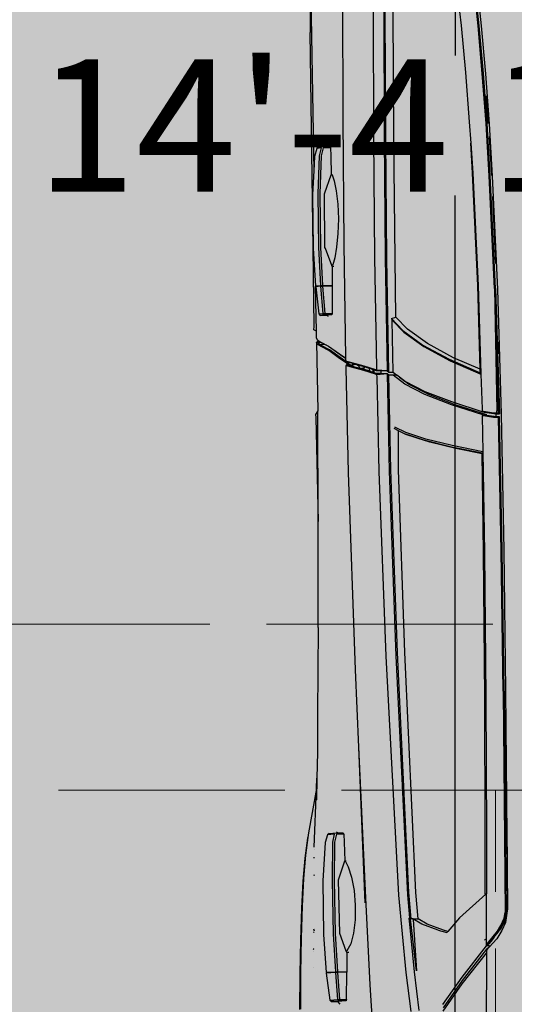
# Model space of a CAD drawing. Units: inches. Extents: x 1884 to 2398, y 474 to 1488.
# Tile 23 of 39: x 2275 to 2301, y 620 to 672. Entities that reach past the tile are written whole.
import ezdxf

# ---------------------------------------------------------------- set-up
doc = ezdxf.new("R2010")
doc.units = ezdxf.units.IN
doc.header["$MEASUREMENT"] = 0
doc.linetypes.add('ACAD_ISO02W100', pattern=[15, 12, -3])
doc.layers.get('0').update_dxf_attribs({"color": 250})
for name, color, linetype, lineweight in [('A-ANNO-DIMS', 2, 'Continuous', 18), ('A-FLOR-OVHD', 8, 'ACAD_ISO02W100', 18), ('C-VEHI', 8, 'Continuous', 18)]:
    doc.layers.add(name, color=color, linetype=linetype, lineweight=lineweight)
doc.layers.add('Edges', color=250, linetype='Continuous')
doc.layers.add('L-PVMT-PATT', color=9, linetype='Continuous', lineweight=13, true_color=0xc7c8ca)
doc.styles.get("Standard").update_dxf_attribs({"font": 'arial.ttf'})
doc.dimstyles.get("Standard").update_dxf_attribs({"dimtxt": 7, "dimasz": 0.18, "dimexe": 0.18, "dimexo": 0.0625, "dimgap": 0.09, "dimtad": 0, "dimtih": 1, "dimtoh": 1, "dimzin": 0, "dimdsep": 46, "dimlunit": 3, "dimtxsty": 'Standard', "dimcen": 0.09, "dimadec": 0, "dimazin": 0, "dimtfac": 1, "dimtofl": 0, "dimtmove": 0, "dimatfit": 3, "dimfxl": 1, "dimtolj": 1, "dimtzin": 0, "dimarcsym": 0})

# ---------------------------------------------------------------- blocks, each defined once
blk = doc.blocks.new('Nissan Qashqai pl')
at = {"layer": 'Edges'}
for p, q in [((9.696, 11.2932), (9.8644, 11.2982)), ((9.8644, 11.2982), (10.0472, 11.3018)), ((10.0476, 11.2996), (9.8681, 11.2959)), ((10.0477, 11.2982), (9.869, 11.2946)), ((10.0472, 11.3018), (10.2357, 11.3043)), ((10.2367, 11.3022), (10.0476, 11.2996)), ((10.2369, 11.3008), (10.0477, 11.2982)), ((10.2357, 11.3043), (10.53, 11.3068)), ((10.2367, 11.3022), (10.5351, 11.305)), ((10.2369, 11.3008), (10.5348, 11.3036)), ((10.4153, 11.3058), (10.2954, 11.3046)), ((10.4153, 11.3058), (10.4174, 11.3058)), ((10.4174, 11.3058), (10.4181, 11.3058)), ((10.4181, 11.3058), (10.4182, 11.3058)), ((10.4182, 11.3058), (10.53, 11.3068)), ((10.53, 11.3068), (10.5301, 11.3068)), ((10.5301, 11.3068), (10.5323, 11.3065)), ((10.5323, 11.3065), (10.5419, 11.3051)), ((10.5422, 11.3021), (10.5348, 11.3036)), ((10.5424, 11.3035), (10.5351, 11.305)), ((10.5366, 11.3048), (10.536, 11.305)), ((10.5379, 11.3052), (10.5381, 11.305)), ((10.5419, 11.3051), (10.5463, 11.3031)), ((10.5419, 11.3051), (10.5479, 11.3042)), ((10.5522, 11.2977), (10.5422, 11.3021)), ((10.5472, 11.3014), (10.5424, 11.3035)), ((10.5463, 11.3031), (10.5551, 11.2984)), ((10.5546, 11.2982), (10.5472, 11.3014)), ((10.5479, 11.3042), (10.5589, 11.2991)), ((10.5598, 11.2935), (10.5522, 11.2977)), ((10.5583, 11.296), (10.5546, 11.2982)), ((10.5551, 11.2984), (10.5583, 11.296)), ((10.5589, 11.2991), (10.57, 11.2925)), ((9.5438, 11.2836), (9.4736, 11.2793)), ((9.4739, 11.282), (9.5443, 11.2863)), ((9.491, 11.2819), (9.5434, 11.2852)), ((9.6953, 11.2892), (9.5437, 11.2822)), ((9.6954, 11.2907), (9.5438, 11.2836)), ((9.5443, 11.2863), (9.696, 11.2932)), ((9.5717, 11.2865), (9.6618, 11.2907)), ((9.6953, 11.2892), (9.863, 11.2944)), ((9.6953, 11.2892), (9.8598, 11.2925)), ((9.6954, 11.2907), (9.8641, 11.2959)), ((9.7669, 11.2945), (9.7832, 11.2951)), ((9.8629, 11.2925), (9.8598, 11.2925)), ((9.8605, 11.2746), (9.8626, 11.2878)), ((9.8615, 11.2754), (9.8635, 11.2886)), ((9.8626, 11.2878), (9.8627, 11.2909)), ((9.8627, 11.2909), (9.8629, 11.2925)), ((9.8627, 11.2909), (9.8637, 11.291)), ((9.8629, 11.2925), (9.863, 11.2944)), ((9.8641, 11.2959), (9.863, 11.2944)), ((9.8635, 11.2886), (9.8637, 11.291)), ((9.8637, 11.291), (9.8638, 11.2934)), ((9.8637, 11.291), (9.8643, 11.291)), ((9.8638, 11.2934), (9.8641, 11.2959)), ((9.8643, 11.291), (9.8677, 11.291)), ((9.8675, 11.2887), (9.8655, 11.2754)), ((9.8686, 11.2879), (9.8665, 11.2747)), ((9.8677, 11.291), (9.8675, 11.2887)), ((9.8678, 11.2935), (9.8677, 11.291)), ((9.8681, 11.2959), (9.8678, 11.2935)), ((9.8681, 11.2959), (9.869, 11.2946)), ((9.8689, 11.2927), (9.8686, 11.2879)), ((9.869, 11.2946), (9.8689, 11.2927)), ((10.5612, 11.2944), (10.5583, 11.296)), ((10.5764, 11.28), (10.5598, 11.2935)), ((10.5683, 11.2885), (10.5612, 11.2944)), ((10.5683, 11.2885), (10.573, 11.285)), ((10.575, 11.2829), (10.5683, 11.2885)), ((10.57, 11.2925), (10.5811, 11.2822)), ((10.573, 11.285), (10.5769, 11.2818)), ((9.2801, 11.2648), (9.3418, 11.2713)), ((9.3418, 11.2713), (9.4064, 11.277)), ((9.4062, 11.2729), (9.3418, 11.2671)), ((9.4063, 11.2743), (9.3419, 11.2685)), ((9.4735, 11.2779), (9.4062, 11.2729)), ((9.4736, 11.2793), (9.4063, 11.2743)), ((9.4064, 11.277), (9.4739, 11.282)), ((9.4727, 11.2808), (9.4362, 11.278)), ((9.4727, 11.2808), (9.4732, 11.2808)), ((9.5437, 11.2822), (9.4735, 11.2779)), ((9.8039, 11.27), (9.6912, 11.2667)), ((9.6913, 11.2674), (9.8099, 11.2711)), ((9.8039, 11.27), (9.7884, 11.2343)), ((9.7905, 11.2283), (9.8087, 11.2702)), ((9.7925, 11.2294), (9.8107, 11.2711)), ((9.8087, 11.2702), (9.8039, 11.27)), ((9.8099, 11.2711), (9.8087, 11.2702)), ((9.8099, 11.2711), (9.8107, 11.2711)), ((9.8107, 11.2711), (9.8573, 11.2726)), ((9.8475, 11.2312), (9.8611, 11.2734)), ((9.8652, 11.2788), (9.8516, 11.2363)), ((9.8652, 11.2738), (9.8516, 11.2313)), ((9.8573, 11.2726), (9.8603, 11.2727)), ((9.8603, 11.2727), (9.8605, 11.2746)), ((9.8611, 11.2734), (9.8603, 11.2727)), ((9.8612, 11.2735), (9.8611, 11.2734)), ((9.8612, 11.2735), (9.8615, 11.2754)), ((9.8652, 11.2738), (9.8652, 11.2788)), ((9.8655, 11.2754), (9.8652, 11.2738)), ((9.8652, 11.2735), (9.8665, 11.2747)), ((9.8652, 11.2738), (9.8652, 11.2738)), ((9.8652, 11.2738), (9.8652, 11.2735)), ((9.8652, 11.2735), (9.8664, 11.2728)), ((9.8665, 11.2747), (9.8664, 11.2728)), ((9.8664, 11.2728), (9.9149, 11.2736)), ((9.9149, 11.2736), (9.9066, 11.2322)), ((9.9169, 11.2728), (9.9086, 11.2313)), ((9.9177, 11.2728), (9.9106, 11.2373)), ((9.9149, 11.2736), (10.0505, 11.276)), ((9.9177, 11.2728), (9.9169, 11.2728)), ((10.0501, 11.2747), (9.9177, 11.2728)), ((10.2453, 11.2762), (10.0501, 11.2747)), ((10.0505, 11.276), (10.2453, 11.2777)), ((10.2453, 11.2777), (10.4289, 11.2783)), ((10.4292, 11.2767), (10.2453, 11.2762)), ((10.4289, 11.2783), (10.5092, 11.2783)), ((10.5099, 11.2768), (10.4292, 11.2767)), ((10.5099, 11.2768), (10.5092, 11.2783)), ((10.5092, 11.2783), (10.5094, 11.2783)), ((10.5094, 11.2783), (10.51, 11.2776)), ((10.5783, 11.2783), (10.5094, 11.2783)), ((10.51, 11.2776), (10.5099, 11.2768)), ((10.51, 11.2776), (10.5419, 11.2423)), ((10.5705, 11.2771), (10.5709, 11.2767)), ((10.5709, 11.2767), (10.5719, 11.2759)), ((10.5776, 11.2808), (10.575, 11.2829)), ((10.5783, 11.2783), (10.5764, 11.28)), ((10.5796, 11.2787), (10.5776, 11.2808)), ((10.5776, 11.2808), (10.5783, 11.2783)), ((10.5796, 11.2787), (10.5783, 11.2783)), ((10.5796, 11.2824), (10.5796, 11.2787)), ((10.6215, 11.2456), (10.5796, 11.2787)), ((10.5811, 11.2822), (10.5821, 11.2808)), ((10.5811, 11.2822), (10.5834, 11.28)), ((10.5821, 11.2808), (10.5834, 11.2793)), ((10.5825, 11.2806), (10.5834, 11.2793)), ((10.5834, 11.28), (10.5851, 11.2783)), ((10.5834, 11.2793), (10.5835, 11.2793)), ((10.5835, 11.2793), (10.584, 11.2787)), ((10.584, 11.2789), (10.584, 11.2793)), ((10.584, 11.2787), (10.584, 11.2789)), ((10.584, 11.2787), (10.6261, 11.2458)), ((10.584, 11.2787), (10.5851, 11.2783)), ((10.5843, 11.2787), (10.584, 11.2787)), ((10.5847, 11.2787), (10.5843, 11.2787)), ((10.5851, 11.2783), (10.5892, 11.2783)), ((10.6306, 11.2459), (10.5892, 11.2783)), ((10.5892, 11.2783), (10.6988, 11.2779)), ((9.3418, 11.2671), (9.2803, 11.2606)), ((9.3419, 11.2685), (9.2804, 11.262)), ((9.471, 11.2554), (9.4997, 11.2573)), ((9.4997, 11.2573), (9.5403, 11.26)), ((9.5404, 11.2598), (9.4997, 11.2573)), ((9.5403, 11.26), (9.6913, 11.2674)), ((9.6912, 11.2667), (9.5404, 11.2598)), ((9.2814, 11.2377), (9.3416, 11.2442)), ((9.3416, 11.2442), (9.4048, 11.2501)), ((9.4048, 11.2501), (9.471, 11.2554)), ((10.6583, 11.2197), (10.6215, 11.2456)), ((10.6261, 11.2458), (10.6627, 11.22)), ((10.6671, 11.2203), (10.6306, 11.2459)), ((9.7884, 11.2343), (9.7692, 11.1989)), ((9.8338, 11.1956), (9.8475, 11.2312)), ((9.8516, 11.2363), (9.8378, 11.2007)), ((9.8516, 11.2313), (9.8378, 11.1957)), ((9.9066, 11.2322), (9.8978, 11.197)), ((9.9086, 11.2313), (9.8998, 11.196)), ((9.9106, 11.2373), (9.9018, 11.2021)), ((10.5419, 11.2423), (10.56, 11.2265)), ((9.7713, 11.1929), (9.7905, 11.2283)), ((9.7733, 11.194), (9.7925, 11.2294)), ((10.5584, 11.2206), (10.5502, 11.1986)), ((10.56, 11.2265), (10.5584, 11.2206)), ((10.5584, 11.2136), (10.5617, 11.2251)), ((10.56, 11.2265), (10.5617, 11.2251)), ((10.5584, 11.2136), (10.5502, 11.1916)), ((9.7692, 11.1989), (9.7499, 11.1721)), ((9.7519, 11.1661), (9.7713, 11.1929)), ((9.754, 11.1672), (9.7733, 11.194)), ((9.8201, 11.1685), (9.8338, 11.1956)), ((9.8378, 11.2007), (9.8241, 11.1736)), ((9.8378, 11.1957), (9.8241, 11.1686)), ((9.8978, 11.197), (9.8891, 11.1701)), ((9.8911, 11.1693), (9.8998, 11.196)), ((9.9018, 11.2021), (9.8931, 11.1752)), ((10.5502, 11.1986), (10.543, 11.1865)), ((10.5502, 11.1916), (10.543, 11.1795)), ((10.5079, 11.1835), (10.1849, 11.1687)), ((10.543, 11.1865), (10.5079, 11.1835)), ((10.543, 11.1795), (10.543, 11.1865)), ((10.5439, 11.1796), (10.543, 11.1795)), ((10.543, 11.1795), (10.543, 11.1771)), ((10.5439, 11.1796), (10.613, 11.1841)), ((10.5458, 11.1742), (10.6144, 11.1813)), ((10.613, 11.1841), (10.547, 11.1767)), ((10.6144, 11.1813), (10.6664, 11.1875)), ((9.7499, 11.1721), (9.7337, 11.1566)), ((9.7357, 11.1507), (9.7519, 11.1661)), ((9.7378, 11.1517), (9.754, 11.1672)), ((9.8241, 11.1686), (9.8119, 11.1529)), ((9.8241, 11.1736), (9.8147, 11.1616)), ((9.8147, 11.1616), (9.8201, 11.1685)), ((9.8891, 11.1701), (9.8818, 11.1551)), ((9.8911, 11.1691), (9.8867, 11.16)), ((9.8931, 11.1751), (9.8911, 11.1693)), ((9.8911, 11.1693), (9.8911, 11.1691)), ((9.8931, 11.1751), (9.8931, 11.1752)), ((10.1849, 11.1687), (9.9393, 11.1602)), ((10.5079, 11.1739), (10.1849, 11.1585)), ((10.1894, 11.1563), (10.5109, 11.1721)), ((10.543, 11.1771), (10.5079, 11.1739)), ((10.5109, 11.1721), (10.5417, 11.1748)), ((10.6152, 11.1702), (10.5113, 11.1603)), ((10.543, 11.1771), (10.5417, 11.1748)), ((10.5417, 11.1748), (10.5427, 11.1739)), ((10.5436, 11.1754), (10.5427, 11.1739)), ((10.5427, 11.1739), (10.5458, 11.1742)), ((10.544, 11.1763), (10.543, 11.1771)), ((10.544, 11.1763), (10.5436, 11.1754)), ((10.547, 11.1767), (10.544, 11.1763)), ((10.6678, 11.177), (10.6152, 11.1702)), ((9.4936, 11.1538), (9.3225, 11.1531)), ((9.6552, 11.1554), (9.4936, 11.1538)), ((9.7337, 11.1566), (9.6552, 11.1554)), ((9.7357, 11.1507), (9.7337, 11.1566)), ((9.7357, 11.1507), (9.7378, 11.1517)), ((9.8078, 11.1528), (9.7378, 11.1517)), ((9.8078, 11.1528), (9.8119, 11.1579)), ((9.8078, 11.1471), (9.8078, 11.1528)), ((9.8147, 11.1616), (9.8119, 11.1579)), ((9.8119, 11.1579), (9.8119, 11.1529)), ((9.8119, 11.1529), (9.8119, 11.1472)), ((9.8147, 11.1616), (9.8147, 11.1616)), ((9.8867, 11.16), (9.8838, 11.1541)), ((9.9393, 11.1602), (9.8867, 11.16)), ((10.1849, 11.1585), (9.9393, 11.1497)), ((9.9411, 11.1475), (10.1894, 11.1563)), ((10.5113, 11.1603), (10.19, 11.1433)), ((9.3198, 11.1403), (9.4922, 11.1409)), ((9.4936, 11.1428), (9.3225, 11.1421)), ((9.4922, 11.1409), (9.654, 11.1423)), ((9.6552, 11.1445), (9.4936, 11.1428)), ((9.654, 11.1423), (9.8061, 11.1447)), ((9.8078, 11.1471), (9.6552, 11.1445)), ((9.8061, 11.1447), (9.8051, 11.1309)), ((9.8058, 11.1369), (9.8061, 11.1447)), ((9.8061, 11.1447), (9.8078, 11.1471)), ((9.8101, 11.1449), (9.8098, 11.1369)), ((9.8101, 11.1449), (9.9411, 11.1475)), ((9.8119, 11.1472), (9.8101, 11.1449)), ((9.8101, 11.1449), (9.8112, 11.1311)), ((9.9393, 11.1497), (9.8119, 11.1472)), ((10.19, 11.1433), (9.9414, 11.1341)), ((9.4919, 11.1269), (9.3194, 11.1262)), ((9.6538, 11.1284), (9.4919, 11.1269)), ((9.802, 11.1309), (9.6538, 11.1284)), ((9.7992, 11.1133), (9.8044, 11.129)), ((9.8051, 11.1309), (9.802, 11.1309)), ((9.8026, 11.1212), (9.8041, 11.1256)), ((9.8041, 11.1256), (9.8045, 11.1268)), ((9.8041, 11.1256), (9.8081, 11.1256)), ((9.8044, 11.129), (9.8051, 11.1309)), ((9.8045, 11.1268), (9.8046, 11.1271)), ((9.8045, 11.1268), (9.8085, 11.1268)), ((9.8046, 11.1271), (9.8055, 11.1298)), ((9.8086, 11.1271), (9.8046, 11.1271)), ((9.8106, 11.1292), (9.8054, 11.1135)), ((9.8055, 11.1298), (9.8058, 11.1369)), ((9.8098, 11.1369), (9.8058, 11.1369)), ((9.8081, 11.1256), (9.8067, 11.1213)), ((9.8085, 11.1268), (9.8081, 11.1256)), ((9.8086, 11.1271), (9.8085, 11.1268)), ((9.8096, 11.13), (9.8086, 11.1271)), ((9.8098, 11.1369), (9.8096, 11.13)), ((9.8112, 11.1311), (9.8106, 11.1292)), ((9.8143, 11.1312), (9.8112, 11.1311)), ((9.9414, 11.1341), (9.8143, 11.1312)), ((10.6318, 11.1213), (10.6955, 11.1257)), ((9.7937, 11.0918), (9.7992, 11.1133)), ((9.7987, 11.108), (9.8002, 11.1141)), ((9.8054, 11.1135), (9.7999, 11.0919)), ((9.8002, 11.1141), (9.8008, 11.1157)), ((9.8008, 11.1157), (9.8014, 11.1176)), ((9.8014, 11.1139), (9.8008, 11.1157)), ((9.803, 11.1212), (9.8014, 11.1176)), ((9.8014, 11.1176), (9.8026, 11.1212)), ((9.8043, 11.1139), (9.8014, 11.1139)), ((9.8031, 11.1093), (9.8014, 11.1139)), ((9.803, 11.1212), (9.8026, 11.1212)), ((9.8067, 11.1213), (9.803, 11.1212)), ((9.8043, 11.1139), (9.8031, 11.1093)), ((9.8044, 11.1142), (9.8043, 11.1139)), ((9.8067, 11.1213), (9.8044, 11.1142)), ((10.312, 11.1064), (10.5147, 11.1156)), ((10.312, 11.1064), (10.5214, 11.1149)), ((10.5147, 11.1156), (10.6318, 11.1213)), ((9.7964, 11.0988), (9.7943, 11.0907)), ((9.7964, 11.0988), (9.7973, 11.1023)), ((9.7964, 11.0988), (9.7992, 11.0966)), ((9.7973, 11.1023), (9.7977, 11.1042)), ((9.7977, 11.1033), (9.7973, 11.1023)), ((9.7973, 11.1023), (9.7977, 11.1011)), ((9.7987, 11.1053), (9.7977, 11.1033)), ((9.7977, 11.1042), (9.7978, 11.1044)), ((9.7977, 11.1042), (9.7977, 11.1033)), ((9.7977, 11.1011), (9.7977, 11.0998)), ((9.7977, 11.1011), (9.7985, 11.099)), ((9.7977, 11.0998), (9.7985, 11.099)), ((9.7978, 11.1044), (9.7987, 11.108)), ((9.7987, 11.1053), (9.7978, 11.1044)), ((9.7985, 11.099), (9.7989, 11.098)), ((9.7992, 11.1065), (9.7987, 11.108)), ((9.7992, 11.1065), (9.7987, 11.1053)), ((9.7989, 11.098), (9.7998, 11.0976)), ((9.8027, 11.1078), (9.7992, 11.1065)), ((9.8002, 11.098), (9.7996, 11.0966)), ((9.8003, 11.0983), (9.7998, 11.0976)), ((9.8002, 11.098), (9.8001, 11.0974)), ((9.8003, 11.0983), (9.8002, 11.098)), ((9.8027, 11.1078), (9.8003, 11.0983)), ((9.8031, 11.1093), (9.8027, 11.1078)), ((9.9426, 11.0923), (10.2081, 11.1017)), ((10.2081, 11.1017), (10.312, 11.1064)), ((10.4871, 11.0967), (10.5048, 11.1002)), ((10.5048, 11.1002), (10.5246, 11.1019)), ((10.5246, 11.1019), (10.5445, 11.1017)), ((10.5445, 11.1017), (10.5625, 11.0996)), ((10.5625, 11.0996), (10.5769, 11.0957)), ((9.2886, 11.0848), (9.4673, 11.0852)), ((9.4673, 11.0852), (9.6358, 11.0866)), ((9.6358, 11.0866), (9.7887, 11.0889)), ((9.7832, 11.0805), (9.7887, 11.0889)), ((9.7842, 11.0814), (9.7891, 11.0889)), ((9.7933, 11.0892), (9.7883, 11.0815)), ((9.7887, 11.0889), (9.7891, 11.0889)), ((9.7891, 11.0889), (9.79, 11.0889)), ((9.7965, 11.0915), (9.7894, 11.0806)), ((9.79, 11.0889), (9.7931, 11.089)), ((9.7931, 11.089), (9.7934, 11.0906)), ((9.7931, 11.089), (9.7933, 11.0892)), ((9.7933, 11.0892), (9.7941, 11.0901)), ((9.7934, 11.0906), (9.7937, 11.0918)), ((9.7934, 11.0906), (9.7938, 11.0904)), ((9.7941, 11.0901), (9.7943, 11.0907)), ((9.7955, 11.0925), (9.7943, 11.0907)), ((9.7963, 11.0918), (9.7955, 11.0925)), ((9.7992, 11.0966), (9.7963, 11.0918)), ((9.7963, 11.0918), (9.7963, 11.0918)), ((9.7964, 11.0917), (9.7963, 11.0918)), ((9.7964, 11.0917), (9.7996, 11.0966)), ((9.7964, 11.0917), (9.7964, 11.0917)), ((9.7967, 11.0915), (9.7964, 11.0917)), ((9.7965, 11.0915), (9.7967, 11.0915)), ((9.7983, 11.0901), (9.7965, 11.0915)), ((9.7967, 11.0915), (9.7986, 11.0916)), ((9.7977, 11.0907), (9.7967, 11.0915)), ((9.7982, 11.0902), (9.7977, 11.0907)), ((9.7986, 11.0916), (9.7982, 11.0902)), ((9.7983, 11.0901), (9.7982, 11.0902)), ((9.7986, 11.0898), (9.7983, 11.0901)), ((9.7988, 11.0925), (9.7986, 11.0916)), ((9.7986, 11.0898), (9.7993, 11.0891)), ((9.7998, 11.0964), (9.7988, 11.0925)), ((9.7998, 11.0976), (9.7992, 11.0966)), ((9.7999, 11.0919), (9.7993, 11.0891)), ((9.7993, 11.0891), (9.8024, 11.0892)), ((9.8001, 11.0974), (9.7996, 11.0966)), ((9.7996, 11.0966), (9.7998, 11.0964)), ((9.8001, 11.0974), (9.7998, 11.0964)), ((9.8024, 11.0892), (9.9426, 11.0923)), ((10.4274, 11.0767), (10.4275, 11.0856)), ((10.4275, 11.0856), (10.4293, 11.0863)), ((10.4293, 11.0863), (10.4291, 11.0765)), ((10.4293, 11.0863), (10.4398, 11.0868)), ((10.4398, 11.0868), (10.4653, 11.0878)), ((10.4653, 11.0881), (10.4652, 11.0897)), ((10.4653, 11.0881), (10.4732, 11.0925)), ((10.4653, 11.0877), (10.4653, 11.0881)), ((10.4653, 11.0878), (10.4653, 11.0881)), ((10.4653, 11.0881), (10.4653, 11.0881)), ((10.4653, 11.0877), (10.4653, 11.0878)), ((10.4908, 11.0793), (10.4653, 11.0877)), ((10.4732, 11.0925), (10.4871, 11.0967)), ((10.5867, 11.0897), (10.563, 11.0809)), ((10.5769, 11.0957), (10.5863, 11.0904)), ((10.5863, 11.0904), (10.5867, 11.0897)), ((10.5885, 11.0904), (10.5867, 11.0897)), ((10.5885, 11.0931), (10.5885, 11.0904)), ((10.5885, 11.0904), (10.6141, 11.0905)), ((10.6141, 11.0905), (10.615, 11.0905)), ((10.6142, 11.0782), (10.6141, 11.0905)), ((10.6517, 11.0902), (10.615, 11.0905)), ((10.615, 11.0905), (10.6151, 11.0782)), ((10.6518, 11.0808), (10.6517, 11.0902)), ((10.6517, 11.0902), (10.6535, 11.0895)), ((10.6535, 11.0895), (10.6543, 11.0786)), ((10.6535, 11.0895), (10.6536, 11.0803)), ((9.5422, 11.0706), (9.5422, 11.0716)), ((9.5424, 11.0707), (9.5503, 11.0736)), ((9.5503, 11.0736), (9.5641, 11.076)), ((9.5641, 11.076), (9.5818, 11.0782)), ((9.5818, 11.0782), (9.6016, 11.0791)), ((9.6016, 11.0791), (9.6215, 11.0782)), ((9.6215, 11.0782), (9.6395, 11.0766)), ((9.6395, 11.0766), (9.654, 11.0744)), ((9.654, 11.0744), (9.6633, 11.0715)), ((9.6633, 11.0715), (9.6645, 11.0705)), ((9.6655, 11.0728), (9.6655, 11.0708)), ((9.7728, 11.066), (9.7832, 11.0805)), ((9.7738, 11.067), (9.7842, 11.0814)), ((9.7883, 11.0815), (9.7778, 11.0671)), ((9.7894, 11.0806), (9.7788, 11.0661)), ((10.4263, 11.0777), (10.4274, 11.0767)), ((10.4274, 11.0762), (10.4274, 11.0767)), ((10.4282, 11.0666), (10.4274, 11.0762)), ((10.4291, 11.0765), (10.4398, 11.0741)), ((10.4398, 11.0718), (10.4291, 11.0741)), ((10.4291, 11.0741), (10.4299, 11.0644)), ((10.4398, 11.0741), (10.4909, 11.0734)), ((10.4909, 11.0711), (10.4398, 11.0718)), ((10.563, 11.0809), (10.4908, 11.0793)), ((10.4909, 11.0734), (10.563, 11.075)), ((10.5631, 11.0727), (10.4909, 11.0711)), ((10.563, 11.075), (10.6142, 11.0779)), ((10.6142, 11.0756), (10.5631, 11.0727)), ((10.6142, 11.0779), (10.6142, 11.0782)), ((10.6142, 11.0765), (10.6142, 11.0779)), ((10.615, 11.0765), (10.6142, 11.0765)), ((10.6142, 11.0756), (10.6142, 11.0765)), ((10.615, 11.0639), (10.6142, 11.0756)), ((10.6151, 11.0765), (10.615, 11.0765)), ((10.615, 11.0765), (10.6151, 11.0639)), ((10.6151, 11.078), (10.6518, 11.0808)), ((10.6518, 11.0784), (10.6151, 11.0756)), ((10.6151, 11.0782), (10.6151, 11.078)), ((10.6151, 11.078), (10.6151, 11.0765)), ((10.6151, 11.0765), (10.6151, 11.0756)), ((10.6151, 11.0756), (10.616, 11.0629)), ((10.6518, 11.0784), (10.6518, 11.0808)), ((10.6518, 11.0808), (10.6536, 11.0803)), ((10.6536, 11.0803), (10.6518, 11.0784)), ((10.6526, 11.0674), (10.6518, 11.0784)), ((10.6536, 11.0803), (10.6537, 11.0783)), ((10.6543, 11.0786), (10.6537, 11.0783)), ((10.6537, 11.0783), (10.6543, 11.0693)), ((10.6578, 11.0814), (10.6543, 11.0786)), ((10.6543, 11.0693), (10.6543, 11.0786)), ((9.5037, 11.0635), (9.5045, 11.0628)), ((9.5044, 11.0586), (9.5045, 11.0628)), ((9.5052, 11.0524), (9.5044, 11.0586)), ((9.5045, 11.0683), (9.5063, 11.0687)), ((9.5045, 11.0628), (9.5045, 11.0683)), ((9.5063, 11.0687), (9.5061, 11.0586)), ((9.5061, 11.0586), (9.5167, 11.0559)), ((9.5063, 11.0687), (9.5168, 11.0691)), ((9.5168, 11.0691), (9.5423, 11.0696)), ((9.5422, 11.0706), (9.5424, 11.0707)), ((9.5423, 11.0696), (9.5422, 11.0706)), ((9.5426, 11.0695), (9.5423, 11.0696)), ((9.5426, 11.0695), (9.5424, 11.0707)), ((9.5667, 11.0609), (9.5426, 11.0695)), ((9.5678, 11.0604), (9.5667, 11.0609)), ((9.5846, 11.0606), (9.5678, 11.0604)), ((9.6236, 11.0609), (9.5846, 11.0606)), ((9.64, 11.0611), (9.6236, 11.0609)), ((9.6413, 11.0616), (9.64, 11.0611)), ((9.6645, 11.0705), (9.6413, 11.0616)), ((9.6655, 11.0708), (9.6645, 11.0705)), ((9.6655, 11.0708), (9.6911, 11.0709)), ((9.6911, 11.0709), (9.692, 11.0709)), ((9.6911, 11.0645), (9.6911, 11.0709)), ((9.6912, 11.0631), (9.6911, 11.0645)), ((9.692, 11.0631), (9.6912, 11.0631)), ((9.6912, 11.0577), (9.6912, 11.0631)), ((9.692, 11.0709), (9.692, 11.0645)), ((9.692, 11.0709), (9.7287, 11.0708)), ((9.692, 11.0645), (9.692, 11.0631)), ((9.692, 11.0631), (9.6921, 11.0578)), ((9.6921, 11.0578), (9.7288, 11.0609)), ((9.7288, 11.0588), (9.6922, 11.0556)), ((9.7287, 11.0708), (9.7305, 11.0704)), ((9.7288, 11.0609), (9.7287, 11.0708)), ((9.7288, 11.0588), (9.7288, 11.0609)), ((9.7288, 11.0609), (9.7306, 11.0607)), ((9.7306, 11.0607), (9.7288, 11.0588)), ((9.7296, 11.0527), (9.7288, 11.0588)), ((9.7305, 11.0704), (9.7313, 11.0644)), ((9.7305, 11.0704), (9.7306, 11.0607)), ((9.7306, 11.0607), (9.7314, 11.0547)), ((9.733, 11.066), (9.7313, 11.0644)), ((9.7314, 11.0547), (9.7313, 11.0644)), ((9.7674, 11.0557), (9.7728, 11.066)), ((9.7684, 11.0567), (9.7717, 11.0631)), ((9.7717, 11.0631), (9.7707, 11.0593)), ((9.7707, 11.0593), (9.7709, 11.0549)), ((9.7717, 11.0631), (9.7738, 11.067)), ((9.7778, 11.0671), (9.7724, 11.0568)), ((9.7788, 11.0661), (9.7734, 11.0558)), ((10.4282, 11.0666), (10.4299, 11.0644)), ((10.4299, 11.0644), (10.4406, 11.0612)), ((10.4406, 11.0612), (10.4919, 11.0584)), ((10.4919, 11.0584), (10.564, 11.0591)), ((10.564, 11.0591), (10.6151, 11.0628)), ((10.6151, 11.0639), (10.615, 11.0639)), ((10.6151, 11.0628), (10.615, 11.0639)), ((10.6151, 11.0639), (10.6151, 11.0628)), ((10.616, 11.0629), (10.6526, 11.0674)), ((10.6526, 11.0674), (10.6543, 11.0693)), ((9.2517, 11.0411), (9.5372, 11.0459)), ((9.641, 11.045), (9.351, 11.0411)), ((9.5052, 11.0524), (9.5069, 11.0501)), ((9.5168, 11.0537), (9.5061, 11.0564)), ((9.5061, 11.0564), (9.5069, 11.0501)), ((9.5069, 11.0501), (9.5176, 11.0469)), ((9.5167, 11.0559), (9.5679, 11.0543)), ((9.5679, 11.0521), (9.5168, 11.0537)), ((9.5176, 11.0469), (9.5372, 11.0459)), ((9.5372, 11.0459), (9.5689, 11.0442)), ((9.5679, 11.0543), (9.64, 11.0549)), ((9.6401, 11.0528), (9.5679, 11.0521)), ((9.5689, 11.0442), (9.641, 11.045)), ((9.64, 11.0549), (9.6912, 11.0577)), ((9.6913, 11.0556), (9.6401, 11.0528)), ((9.641, 11.045), (9.6921, 11.0485)), ((9.7466, 11.0464), (9.641, 11.045)), ((9.6913, 11.0556), (9.6912, 11.0577)), ((9.692, 11.0499), (9.6913, 11.0556)), ((9.6922, 11.0499), (9.692, 11.0499)), ((9.6921, 11.0485), (9.692, 11.0499)), ((9.6922, 11.0556), (9.6921, 11.0578)), ((9.6922, 11.0499), (9.6921, 11.0485)), ((9.7526, 11.0495), (9.6921, 11.0485)), ((9.6922, 11.0556), (9.693, 11.0486)), ((9.6922, 11.0556), (9.6922, 11.0499)), ((9.693, 11.0486), (9.7296, 11.0527)), ((9.7296, 11.0527), (9.7314, 11.0547)), ((9.7511, 11.0463), (9.7466, 11.0464)), ((9.7526, 11.0495), (9.7511, 11.0463)), ((9.7623, 11.0497), (9.7526, 11.0495)), ((9.7623, 11.0497), (9.7643, 11.0504)), ((9.7643, 11.0504), (9.7652, 11.0514)), ((9.7643, 11.0504), (9.7648, 11.0513)), ((9.7648, 11.0513), (9.7664, 11.054)), ((9.7648, 11.0513), (9.7648, 11.0513)), ((9.7652, 11.0514), (9.7665, 11.0535)), ((9.7664, 11.054), (9.7674, 11.0557)), ((9.7665, 11.0537), (9.7664, 11.054)), ((9.7665, 11.0535), (9.7676, 11.0553)), ((9.7667, 11.0508), (9.7665, 11.0535)), ((9.7676, 11.0511), (9.7667, 11.0508)), ((9.7677, 11.0498), (9.7667, 11.0508)), ((9.7673, 11.0545), (9.7676, 11.0553)), ((9.7673, 11.0543), (9.7673, 11.0545)), ((9.7676, 11.0511), (9.7673, 11.0543)), ((9.7676, 11.0553), (9.7684, 11.0567)), ((9.7676, 11.0555), (9.7678, 11.056)), ((9.769, 11.0516), (9.7676, 11.0511)), ((9.7677, 11.0498), (9.8598, 11.0514)), ((9.77, 11.0506), (9.7677, 11.0498)), ((9.7677, 11.0498), (9.7677, 11.0498)), ((9.7712, 11.055), (9.769, 11.0516)), ((9.7734, 11.0558), (9.77, 11.0506)), ((9.7709, 11.0549), (9.7712, 11.055)), ((9.7724, 11.0568), (9.7712, 11.055)), ((9.8598, 11.0514), (9.8614, 11.0504)), ((9.8643, 11.0514), (9.8598, 11.0514)), ((9.8614, 11.0504), (9.8647, 11.0485)), ((10.0085, 11.0519), (9.8643, 11.0514)), ((9.8647, 11.0485), (9.869, 11.0488)), ((9.869, 11.0488), (10.0085, 11.0519)), ((10.0124, 11.0519), (10.0085, 11.0519)), ((10.1513, 11.0517), (10.0124, 11.0519)), ((10.1513, 11.0517), (10.2677, 11.0512)), ((10.2677, 11.0512), (10.3189, 11.0511)), ((10.3189, 11.0511), (10.3537, 11.0503)), ((10.3537, 11.0503), (10.3832, 11.0496)), ((10.3679, 11.0497), (10.3537, 11.0503)), ((10.3679, 11.0497), (10.4275, 11.0391)), ((10.4468, 11.0466), (10.3679, 11.0497)), ((10.4502, 11.0466), (10.4503, 11.0465)), ((10.4613, 11.0464), (10.4603, 11.0465)), ((10.4838, 11.0465), (10.4852, 11.046)), ((10.5565, 11.0456), (10.5591, 11.0464)), ((10.5615, 11.0464), (10.5617, 11.0457)), ((10.583, 11.0457), (10.5835, 11.0461)), ((10.5836, 11.0461), (10.5832, 11.0457)), ((10.5847, 11.0461), (10.5841, 11.0457)), ((10.5873, 11.0461), (10.5873, 11.0461)), ((10.6087, 11.0458), (10.6087, 11.0458)), ((9.2517, 11.0411), (9.351, 11.0411)), ((10.4275, 11.0391), (10.4304, 11.0385)), ((10.4304, 11.0385), (10.4339, 11.0381)), ((10.4345, 11.0379), (10.4339, 11.0381)), ((10.4339, 11.0381), (10.4573, 11.0349)), ((10.4613, 11.0343), (10.4345, 11.0379)), ((10.4573, 11.0349), (10.4889, 11.0323)), ((10.4926, 11.0317), (10.4613, 11.0343)), ((10.4889, 11.0323), (10.526, 11.0304)), ((10.5294, 11.0298), (10.4926, 11.0317)), ((10.526, 11.0304), (10.569, 11.0291)), ((10.5719, 11.0285), (10.5294, 11.0298)), ((10.569, 11.0291), (10.5919, 11.0287)), ((10.6176, 11.0277), (10.5719, 11.0285)), ((10.5919, 11.0287), (10.5936, 11.0286)), ((10.5936, 11.0286), (10.6151, 11.0283)), ((10.6151, 11.0283), (10.6644, 11.028)), ((10.6651, 11.0274), (10.6176, 11.0277))]:
    blk.add_line(p, q, dxfattribs=at)
blk = doc.blocks.new('car')
blk.add_blockref('Nissan Qashqai pl', (-9.7433, -11.9151))
blk = doc.blocks.new('carr')
blk.add_blockref('car', (0.5124, -0.007))
blk = doc.blocks.new('*D23')
at = {"layer": 'A-ANNO-DIMS', "color": 0, "lineweight": -2, "transparency": 16777216}
for p, q in [((2272.304, 752.812), (2298.291, 752.812)), ((2298.111, 752.632), (2298.111, 670.29)), ((2298.111, 580.529), (2298.111, 662.871)), ((2272.304, 580.349), (2298.291, 580.349))]:
    blk.add_line(p, q, dxfattribs=at)
at = {"layer": 'A-ANNO-DIMS', "color": 0, "lineweight": 100, "transparency": 16777216}
for points in [[(2298.081, 752.632), (2298.141, 752.632), (2298.111, 752.812)], [(2298.081, 580.529), (2298.141, 580.529), (2298.111, 580.349)]]:
    blk.add_solid(points, dxfattribs=at)
at = {"layer": 'Defpoints', "color": 0, "lineweight": 100, "transparency": 16777216}
for p in [(2272.242, 752.812), (2272.242, 580.349), (2298.111, 580.349)]:
    blk.add_point(p, dxfattribs=at)
at = {"layer": 'A-ANNO-DIMS', "color": 0, "transparency": 16777216, "insert": (2298.111, 666.58), "char_height": 7, "attachment_point": 5}
blk.add_mtext('\\A1;CAR 14\'-4 1/2" TYP.', dxfattribs=at)

msp = doc.modelspace()

# ---------------------------------------------------------------- hatches: boundary and pattern name
at = {"layer": 'L-PVMT-PATT'}
h = msp.add_hatch(color=256, dxfattribs=at)
h.dxf.hatch_style = 1
h.paths.add_polyline_path([(2387.529, 769.966), (2351.529, 769.966), (2238.447, 769.966), (2238.447, 762.15), (2238.447, 754.445), (2126.529, 754.445), (2126.529, 676.183), (2134.868, 676.183), (2142.673, 676.183), (2142.673, 646.578), (2134.868, 646.578), (2126.529, 646.578), (2126.529, 640.17), (2387.529, 640.17)])
h.paths.add_polyline_path([(2387.529, 631.385), (2303.086, 631.385), (2303.086, 615.671), (2387.529, 615.671)])
h.paths.add_polyline_path([(2387.529, 640.17), (2126.529, 640.17), (2126.529, 631.385), (2387.529, 631.385)])
h.paths.add_polyline_path([(2393.529, 604.13), (2387.529, 604.13), (2387.529, 615.671), (2303.086, 615.671), (2303.086, 607.943), (2249.649, 607.943), (2126.529, 607.943), (2126.529, 533.885), (2393.529, 533.885)])
h.paths.add_polyline_path([(2257.825, 611.008), (2257.83, 611.337), (2257.915, 616.493), (2258.021, 621.805), (2258.146, 627.274), (2258.252, 631.385), (2126.529, 631.385), (2126.529, 611.008)])
h.paths.add_polyline_path([(2258.892, 611.285), (2258.888, 611.008), (2300.247, 611.008), (2300.247, 631.385), (2259.314, 631.385), (2259.206, 627.173), (2259.081, 621.72), (2258.976, 616.424)])
h = msp.add_hatch(color=256, dxfattribs=at)
h.dxf.hatch_style = 1
h.paths.add_polyline_path([(2216.015, 611.008), (2212.351, 611.008), (2212.342, 608.327), (2212.34, 607.943), (2216.046, 607.943), (2216.044, 608.264)])
h.paths.add_polyline_path([(2212.351, 611.008), (2211.081, 611.008), (2210.074, 609.575), (2209.435, 608.376), (2209.305, 607.943), (2212.34, 607.943), (2212.342, 608.327)])
h.paths.add_polyline_path([(2257.742, 611.008), (2249.649, 611.008), (2217.664, 611.008), (2217.692, 608.284), (2217.694, 607.943), (2249.649, 607.943), (2257.712, 607.943), (2257.713, 608.284)])
h.paths.add_polyline_path([(2266.79, 611.008), (2264.592, 611.008), (2265.355, 609.923), (2266.022, 608.672), (2266.241, 607.943), (2266.364, 607.943), (2266.622, 609.602)])
h.paths.add_polyline_path([(2263.055, 611.008), (2259.39, 611.008), (2259.361, 608.264), (2259.359, 607.943), (2263.065, 607.943), (2263.063, 608.327)])
h.paths.add_polyline_path([(2265.331, 609.575), (2264.325, 611.008), (2263.055, 611.008), (2263.063, 608.327), (2263.065, 607.943), (2266.1, 607.943), (2265.97, 608.376)])
h.paths.add_polyline_path([(2272.885, 609.347), (2272.901, 609.457), (2272.902, 609.679), (2272.895, 611.008), (2271.456, 611.008), (2271.351, 610.147), (2271.277, 610.077), (2270.912, 610.081), (2270.481, 610.11), (2270.455, 610.183), (2270.448, 611.008), (2269.23, 611.008), (2269.228, 610.963), (2269.055, 608.458), (2269.014, 607.943), (2272.869, 607.943), (2272.882, 607.958)])
h.paths.add_polyline_path([(2269.228, 610.963), (2269.23, 611.008), (2267.227, 611.008), (2267.038, 609.547), (2266.77, 607.943), (2269.014, 607.943), (2269.055, 608.458)])
h.paths.add_polyline_path([(2293.178, 611.008), (2272.917, 611.008), (2272.925, 609.643), (2272.924, 609.184), (2272.925, 609.03), (2272.921, 607.943), (2293.123, 607.943), (2293.127, 608.565), (2293.159, 610.362)])
h.paths.add_polyline_path([(2302.932, 613.651), (2302.931, 615.98), (2302.91, 623.22), (2302.851, 630.905), (2302.844, 631.385), (2300.247, 631.385), (2300.247, 612.163), (2300.885, 611.925), (2301.121, 611.86), (2301.743, 612.576)])
h.paths.add_polyline_path([(2302.992, 610.861), (2302.993, 612.796), (2302.965, 612.8), (2301.576, 611.546), (2300.954, 610.83), (2300.899, 610.766), (2300.444, 610.894), (2300.139, 611.008), (2299.369, 611.008), (2299.448, 609.776), (2299.311, 611.008), (2299.207, 611.008), (2299.34, 609.722), (2299.553, 607.943), (2300.825, 607.943), (2300.851, 607.993), (2301.87, 609.442)])
h.paths.add_polyline_path([(2298.512, 611.008), (2296.882, 611.008), (2296.979, 609.034), (2297.054, 607.943), (2298.828, 607.943), (2298.736, 608.659)])
h.paths.add_polyline_path([(2294.51, 608.662), (2294.51, 608.662), (2294.362, 610.672), (2294.359, 611.008), (2293.338, 611.008), (2293.331, 610.606), (2293.329, 610.538), (2293.315, 609.691), (2293.305, 607.943), (2294.597, 607.943)])
h.paths.add_polyline_path([(2302.991, 609.68), (2301.718, 608.051), (2301.642, 607.943), (2302.986, 607.943)], flags=17)

# ---------------------------------------------------------------- linework, layer by layer
at = {"layer": 'A-FLOR-OVHD'}
for p, q in [((2258.112, 640.17), (2308.043, 640.17)), ((2262.087, 631.385), (2308.262, 631.385)), ((2300.247, 611.008), (2300.247, 631.385))]:
    msp.add_line(p, q, dxfattribs=at)

# ---------------------------------------------------------------- block references
at = {"layer": 'C-VEHI', "xscale": 39.37007874015748, "yscale": 39.37007874015748, "zscale": 39.37007874015748, "rotation": 270}
msp.add_blockref('carr', (2325.111, 676.232), dxfattribs=at)

# ---------------------------------------------------------------- dimensions: what is measured, and where the dimension line sits
at = {"layer": 'A-ANNO-DIMS'}
dim = msp.add_linear_dim(base=(2298.111, 580.349), p1=(2272.242, 752.812), p2=(2272.242, 580.349), angle=270, text='CAR <> TYP.', dimstyle='Standard', override={"dimdec": 1, "dimlfac": 1, "dimrnd": 0, "dimzin": 1, "dimdsep": 46, "dimlunit": 4, "dimfrac": 2}, dxfattribs=at)
dim.commit()
dim.dimension.update_dxf_attribs({"geometry": '*D23', "text_midpoint": (2298.111, 666.58)})

doc.saveas('drawing.dxf')
